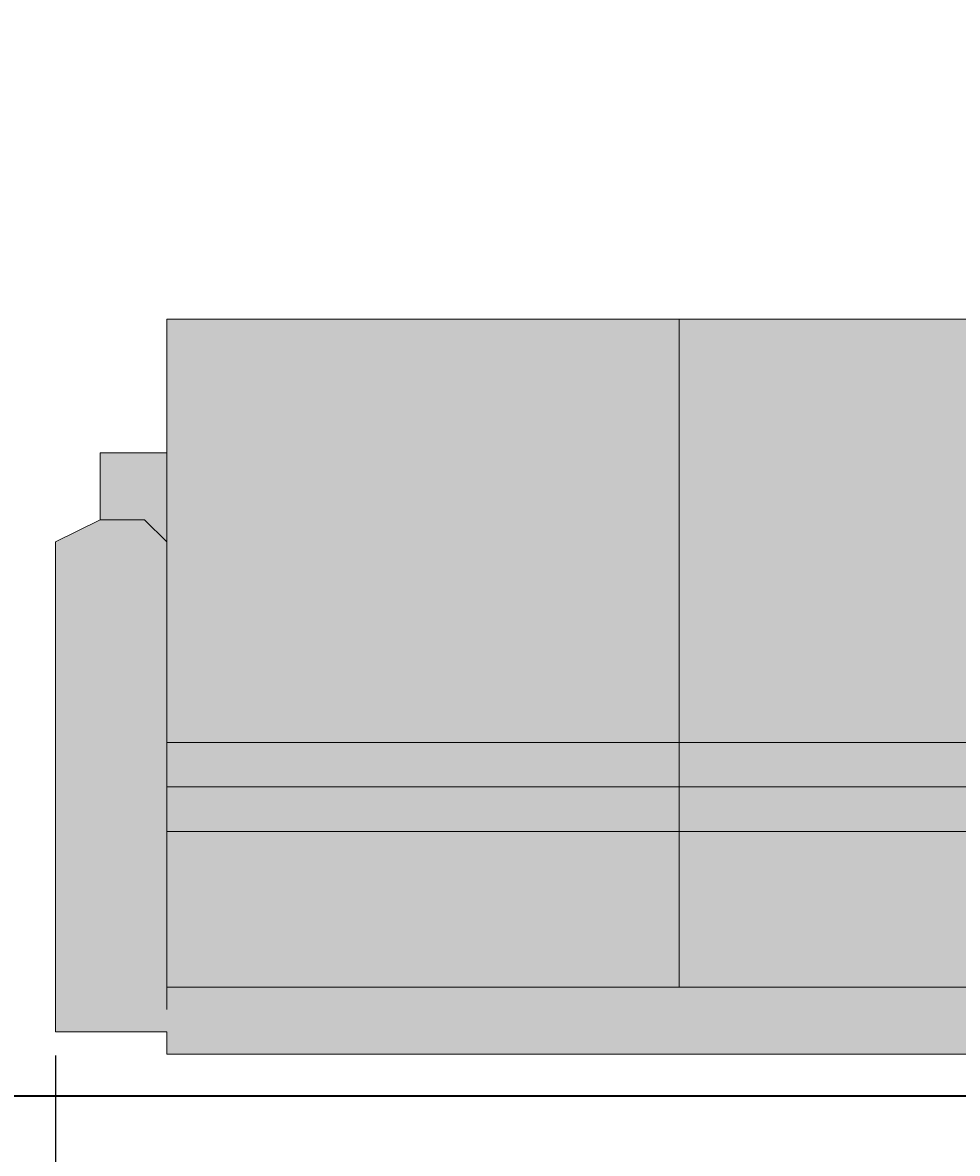
# Model space of a CAD drawing. Units: millimetres. Extents: x 27017497 to 27018854, y 7058029 to 7059154.
# Tile 34 of 91: x 27017677 to 27017714, y 7058297 to 7058341. Entities that reach past the tile are written whole.
import ezdxf

# ---------------------------------------------------------------- set-up
doc = ezdxf.new("R2010")
doc.units = ezdxf.units.MM
for name, color, linetype, lineweight in [('A-ANNO-DIMS', 2, 'Continuous', 18), ('A-FURN', 8, 'Continuous', 18), ('A-WALL', 7, 'Continuous', 35)]:
    doc.layers.add(name, color=color, linetype=linetype, lineweight=lineweight)
doc.layers.add('A-FURN-PATT', color=177, linetype='Continuous', lineweight=13, true_color=0x293189)
doc.styles.get("Standard").update_dxf_attribs({"font": 'arial.ttf'})
doc.dimstyles.get("Standard").update_dxf_attribs({"dimtxt": 0.18, "dimasz": 0.18, "dimexe": 0.18, "dimexo": 0.0625, "dimgap": 0.09, "dimtad": 0, "dimtih": 1, "dimtoh": 1, "dimdec": 4, "dimzin": 0, "dimdsep": 46, "dimtxsty": 'Standard', "dimcen": 0.09, "dimadec": 0, "dimazin": 0, "dimtfac": 1, "dimtdec": 4, "dimtofl": 0, "dimtmove": 0, "dimatfit": 3, "dimfxl": 1, "dimtolj": 1, "dimtzin": 0, "dimarcsym": 0})

# ---------------------------------------------------------------- blocks, each defined once
blk = doc.blocks.new('SOFA-LIVING-THREE-SEAT')
for p, q in [((63.532, 28.72), (4.351, 28.72)), ((4.351, 28.72), (4.351, 23.498)), ((24.368, 28.72), (24.368, 2.611)), ((43.515, 28.72), (43.515, 2.611)), ((63.532, 23.498), (63.532, 28.72)), ((4.351, 23.498), (1.741, 23.498)), ((1.741, 23.498), (1.741, 20.887)), ((4.351, 23.498), (4.351, 20.017)), ((63.532, 23.498), (63.532, 20.017)), ((66.142, 23.498), (63.532, 23.498)), ((66.142, 20.887), (66.142, 23.498)), ((1.741, 20.887), (0, 20.017)), ((1.741, 20.887), (3.481, 20.887)), ((3.481, 20.887), (4.351, 20.017)), ((64.402, 20.887), (63.532, 20.017)), ((66.142, 20.887), (64.402, 20.887)), ((67.883, 20.017), (66.142, 20.887)), ((0, 20.017), (0, 0.871)), ((4.351, 20.017), (4.351, 1.741)), ((63.532, 20.017), (63.532, 1.741)), ((67.883, 0.871), (67.883, 20.017)), ((63.532, 12.184), (4.351, 12.184)), ((63.532, 10.444), (4.351, 10.444)), ((63.532, 8.703), (4.351, 8.703)), ((4.351, 2.611), (63.532, 2.611)), ((0, 0.871), (4.351, 0.871)), ((4.351, 0.871), (4.351, 0)), ((63.532, 0), (63.532, 0.871)), ((63.532, 0.871), (67.883, 0.871)), ((4.351, 0), (63.532, 0))]:
    blk.add_line(p, q)
blk = doc.blocks.new('*D39')
at = {"layer": 'A-ANNO-DIMS', "color": 0, "lineweight": -2, "transparency": 16777216}
for p, q in [((27017678.38, 7058300.482), (27017678.38, 7058290.182)), ((27017746.263, 7058300.482), (27017746.263, 7058290.182)), ((27017678.56, 7058290.362), (27017710.973, 7058290.362)), ((27017746.083, 7058290.362), (27017713.67, 7058290.362))]:
    blk.add_line(p, q, dxfattribs=at)
at = {"layer": 'A-ANNO-DIMS', "color": 0, "transparency": 16777216}
for points in [[(27017678.56, 7058290.392), (27017678.56, 7058290.332), (27017678.38, 7058290.362)], [(27017746.083, 7058290.392), (27017746.083, 7058290.332), (27017746.263, 7058290.362)]]:
    blk.add_solid(points, dxfattribs=at)
at = {"layer": 'Defpoints', "color": 0, "transparency": 16777216}
for p in [(27017678.38, 7058300.544), (27017746.263, 7058300.544), (27017746.263, 7058290.362)]:
    blk.add_point(p, dxfattribs=at)
at = {"layer": 'A-ANNO-DIMS', "color": 0, "transparency": 16777216, "insert": (27017712.321, 7058290.362), "char_height": 0.18, "attachment_point": 5}
blk.add_mtext('\\A1;LIVING SOFA 68 TYP.', dxfattribs=at)
blk = doc.blocks.new('*D48')
at = {"layer": 'A-ANNO-DIMS', "color": 0, "lineweight": -2, "transparency": 16777216}
for p, q in [((27018463.498, 7058622.912), (27017497.536, 7058622.912)), ((27017497.716, 7058622.732), (27017497.716, 7058357.753)), ((27017497.716, 7058092.41), (27017497.716, 7058357.389)), ((27018555.129, 7058092.23), (27017497.536, 7058092.23))]:
    blk.add_line(p, q, dxfattribs=at)
at = {"layer": 'A-ANNO-DIMS', "color": 0, "transparency": 16777216}
for points in [[(27017497.686, 7058622.732), (27017497.746, 7058622.732), (27017497.716, 7058622.912)], [(27017497.686, 7058092.41), (27017497.746, 7058092.41), (27017497.716, 7058092.23)]]:
    blk.add_solid(points, dxfattribs=at)
at = {"layer": 'Defpoints', "color": 0, "transparency": 16777216}
for p in [(27018463.561, 7058622.912), (27017497.716, 7058092.23), (27018555.192, 7058092.23)]:
    blk.add_point(p, dxfattribs=at)
at = {"layer": 'A-ANNO-DIMS', "color": 0, "transparency": 16777216, "insert": (27017497.716, 7058357.571), "char_height": 0.18, "attachment_point": 5}
blk.add_mtext('\\A1;530.7', dxfattribs=at)

msp = doc.modelspace()

# ---------------------------------------------------------------- hatches: boundary and pattern name
at = {"layer": 'A-FURN-PATT'}
h = msp.add_hatch(color=256, dxfattribs=at)
h.dxf.hatch_style = 1
h.paths.add_polyline_path([(27017702.748, 7058329.264), (27017682.731, 7058329.264), (27017682.731, 7058324.042), (27017682.731, 7058320.561), (27017682.731, 7058312.728), (27017702.748, 7058312.728)])
h.paths.add_polyline_path([(27017721.895, 7058329.264), (27017702.748, 7058329.264), (27017702.748, 7058312.728), (27017721.895, 7058312.728)])
h.paths.add_polyline_path([(27017741.912, 7058320.561), (27017741.912, 7058324.042), (27017741.912, 7058329.264), (27017721.895, 7058329.264), (27017721.895, 7058312.728), (27017741.912, 7058312.728)])
h.paths.add_polyline_path([(27017682.731, 7058320.561), (27017681.861, 7058321.431), (27017680.121, 7058321.431), (27017678.38, 7058320.561), (27017678.38, 7058301.415), (27017682.731, 7058301.415), (27017682.731, 7058300.544), (27017741.912, 7058300.544), (27017741.912, 7058301.415), (27017746.263, 7058301.415), (27017746.263, 7058320.561), (27017744.522, 7058321.431), (27017742.782, 7058321.431), (27017741.912, 7058320.561), (27017741.912, 7058303.155), (27017682.731, 7058303.155)])
h.paths.add_polyline_path([(27017741.912, 7058309.247), (27017721.895, 7058309.247), (27017721.895, 7058303.155), (27017741.912, 7058303.155)], flags=17)
h.paths.add_polyline_path([(27017721.895, 7058309.247), (27017702.748, 7058309.247), (27017702.748, 7058303.155), (27017721.895, 7058303.155)], flags=17)
h.paths.add_polyline_path([(27017702.748, 7058309.247), (27017682.731, 7058309.247), (27017682.731, 7058303.155), (27017702.748, 7058303.155)], flags=17)
h.paths.add_polyline_path([(27017702.748, 7058312.728), (27017682.731, 7058312.728), (27017682.731, 7058310.988), (27017702.748, 7058310.988)], flags=17)
h.paths.add_polyline_path([(27017721.895, 7058312.728), (27017702.748, 7058312.728), (27017702.748, 7058310.988), (27017721.895, 7058310.988)], flags=17)
h.paths.add_polyline_path([(27017741.912, 7058312.728), (27017721.895, 7058312.728), (27017721.895, 7058310.988), (27017741.912, 7058310.988)], flags=17)
h.paths.add_polyline_path([(27017741.912, 7058310.988), (27017721.895, 7058310.988), (27017721.895, 7058309.247), (27017741.912, 7058309.247)], flags=17)
h.paths.add_polyline_path([(27017721.895, 7058310.988), (27017702.748, 7058310.988), (27017702.748, 7058309.247), (27017721.895, 7058309.247)], flags=17)
h.paths.add_polyline_path([(27017702.748, 7058310.988), (27017682.731, 7058310.988), (27017682.731, 7058309.247), (27017702.748, 7058309.247)], flags=17)
h.paths.add_polyline_path([(27017744.522, 7058324.042), (27017741.912, 7058324.042), (27017741.912, 7058320.561), (27017742.782, 7058321.431), (27017744.522, 7058321.431)])
h.paths.add_polyline_path([(27017682.731, 7058324.042), (27017680.121, 7058324.042), (27017680.121, 7058321.431), (27017681.861, 7058321.431), (27017682.731, 7058320.561)])

# ---------------------------------------------------------------- linework, layer by layer
at = {"layer": 'A-WALL'}
msp.add_line((27017641.166, 7058298.912), (27017743.666, 7058298.912), dxfattribs=at)

# ---------------------------------------------------------------- block references
at = {"layer": 'A-FURN'}
msp.add_blockref('SOFA-LIVING-THREE-SEAT', (27017678.38, 7058300.544), dxfattribs=at)

# ---------------------------------------------------------------- dimensions: what is measured, and where the dimension line sits
at = {"layer": 'A-ANNO-DIMS'}
dim = msp.add_linear_dim(base=(27017497.716, 7058092.23), p1=(27018463.561, 7058622.912), p2=(27018555.192, 7058092.23), angle=90, dimstyle='Standard', override={"dimdec": 1, "dimlfac": 1, "dimrnd": 0, "dimzin": 0, "dimdsep": 46, "dimlunit": 2}, dxfattribs=at)
dim.commit()
dim.dimension.update_dxf_attribs({"geometry": '*D48', "text_midpoint": (27017497.716, 7058357.571)})
dim = msp.add_linear_dim(base=(27017746.263, 7058290.362), p1=(27017678.38, 7058300.544), p2=(27017746.263, 7058300.544), text='LIVING SOFA <> TYP.', dimstyle='Standard', override={"dimdec": 0, "dimlfac": 1, "dimrnd": 0, "dimzin": 0, "dimdsep": 46, "dimlunit": 2}, dxfattribs=at)
dim.commit()
dim.dimension.update_dxf_attribs({"geometry": '*D39', "text_midpoint": (27017712.321, 7058290.362)})

doc.saveas('drawing.dxf')
